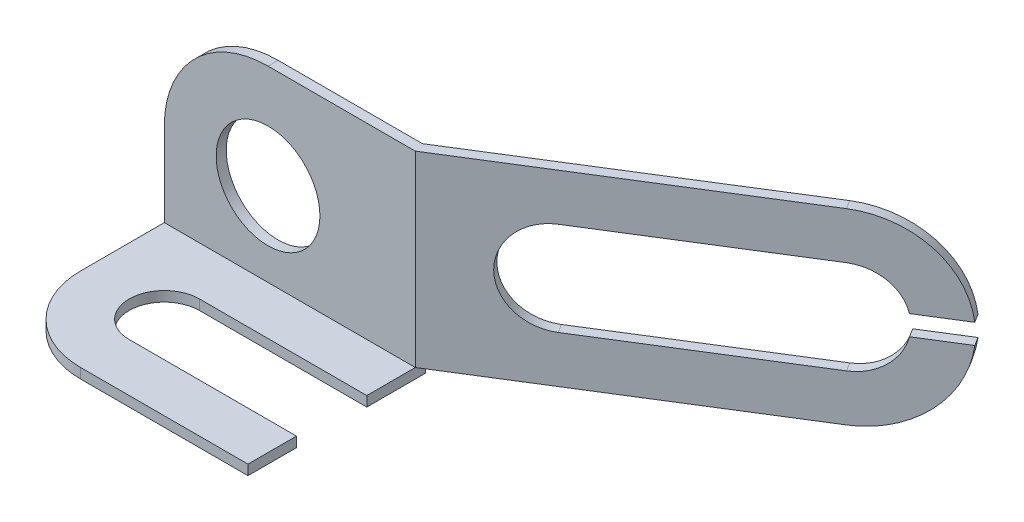
ISO-10303-21;
HEADER;
FILE_DESCRIPTION(('STEP AP214'),'2;1');
FILE_NAME('part.step','',(''),(''),'','','');
FILE_SCHEMA(('AUTOMOTIVE_DESIGN { 1 0 10303 214 1 1 1 1 }'));
ENDSEC;
DATA;
#1=APPLICATION_CONTEXT('core data for automotive mechanical design processes');
#2=APPLICATION_PROTOCOL_DEFINITION('international standard','automotive_design',2000,#1);
#3=PRODUCT_CONTEXT('',#1,'mechanical');
#4=PRODUCT('Part','Part','',(#3));
#5=PRODUCT_RELATED_PRODUCT_CATEGORY('part','',(#4));
#6=PRODUCT_DEFINITION_FORMATION('','',#4);
#7=PRODUCT_DEFINITION_CONTEXT('part definition',#1,'design');
#8=PRODUCT_DEFINITION('design','',#6,#7);
#9=PRODUCT_DEFINITION_SHAPE('','',#8);
#10=(LENGTH_UNIT() NAMED_UNIT(*) SI_UNIT(.MILLI.,.METRE.));
#11=(NAMED_UNIT(*) PLANE_ANGLE_UNIT() SI_UNIT($,.RADIAN.));
#12=(NAMED_UNIT(*) SI_UNIT($,.STERADIAN.) SOLID_ANGLE_UNIT());
#13=UNCERTAINTY_MEASURE_WITH_UNIT(LENGTH_MEASURE(1.E-05),#10,'distance_accuracy_value','');
#14=(GEOMETRIC_REPRESENTATION_CONTEXT(3) GLOBAL_UNCERTAINTY_ASSIGNED_CONTEXT((#13)) GLOBAL_UNIT_ASSIGNED_CONTEXT((#10,
#11,#12)) REPRESENTATION_CONTEXT('',''));
#15=CARTESIAN_POINT('',(0.,0.,0.));
#16=DIRECTION('',(0.,0.,1.));
#17=DIRECTION('',(1.,0.,0.));
#18=AXIS2_PLACEMENT_3D('',#15,#16,#17);
#19=CARTESIAN_POINT('',(1.55405478395852,0.56,-1.04183190988548));
#20=DIRECTION('',(0.529919264233206,0.,0.848048096156425));
#21=DIRECTION('',(0.848048096156426,0.,-0.529919264233206));
#22=AXIS2_PLACEMENT_3D('',#19,#20,#21);
#23=CYLINDRICAL_SURFACE('',#22,0.56);
#24=CARTESIAN_POINT('',(1.55405478395852,0.56,-1.04183190988548));
#25=DIRECTION('',(0.529919264233206,0.,0.848048096156425));
#26=DIRECTION('',(0.848048096156426,0.,-0.529919264233206));
#27=AXIS2_PLACEMENT_3D('',#24,#25,#26);
#28=CIRCLE('',#27,0.56);
#29=CARTESIAN_POINT('',(2.02622798073308,0.5,-1.33687846934296));
#30=VERTEX_POINT('',#29);
#31=CARTESIAN_POINT('',(1.55405478395852,0.,-1.04183190988548));
#32=VERTEX_POINT('',#31);
#33=EDGE_CURVE('E48',#30,#32,#28,.F.);
#34=ORIENTED_EDGE('',*,*,#33,.F.);
#35=DIRECTION('',(0.529919264233206,0.,0.848048096156425));
#36=VECTOR('',#35,1.);
#37=CARTESIAN_POINT('',(2.02622798073308,0.5,-1.33687846934295));
#38=LINE('',#37,#36);
#39=CARTESIAN_POINT('',(2.05802313658707,0.5,-1.28599558357357));
#40=VERTEX_POINT('',#39);
#41=EDGE_CURVE('E93',#30,#40,#38,.T.);
#42=ORIENTED_EDGE('',*,*,#41,.T.);
#43=CARTESIAN_POINT('',(1.58584993981252,0.56,-0.990949024116095));
#44=DIRECTION('',(0.529919264233206,0.,0.848048096156425));
#45=DIRECTION('',(0.848048096156426,0.,-0.529919264233206));
#46=AXIS2_PLACEMENT_3D('',#43,#44,#45);
#47=CIRCLE('',#46,0.56);
#48=CARTESIAN_POINT('',(1.58584993981251,0.,-0.990949024116095));
#49=VERTEX_POINT('',#48);
#50=EDGE_CURVE('E12',#49,#40,#47,.T.);
#51=ORIENTED_EDGE('',*,*,#50,.F.);
#52=DIRECTION('',(0.529919264233206,0.,0.848048096156425));
#53=VECTOR('',#52,1.);
#54=CARTESIAN_POINT('',(1.55405478395852,0.,-1.04183190988548));
#55=LINE('',#54,#53);
#56=EDGE_CURVE('E226',#32,#49,#55,.T.);
#57=ORIENTED_EDGE('',*,*,#56,.F.);
#58=EDGE_LOOP('',(#34,#42,#51,#57));
#59=FACE_BOUND('',#58,.T.);
#60=ADVANCED_FACE('F43',(#59),#23,.T.);
#61=CARTESIAN_POINT('',(-0.0317951558539923,0.,-0.0508828857693855));
#62=DIRECTION('',(-0.529919264233206,0.,-0.848048096156426));
#63=DIRECTION('',(-0.848048096156425,0.,0.529919264233206));
#64=AXIS2_PLACEMENT_3D('',#61,#62,#63);
#65=PLANE('',#64);
#66=CARTESIAN_POINT('',(1.55405478395852,0.56,-1.04183190988548));
#67=DIRECTION('',(0.529919264233206,0.,0.848048096156425));
#68=DIRECTION('',(0.848048096156426,0.,-0.529919264233206));
#69=AXIS2_PLACEMENT_3D('',#66,#67,#68);
#70=CIRCLE('',#69,0.56);
#71=CARTESIAN_POINT('',(1.55405478395852,1.12,-1.04183190988548));
#72=VERTEX_POINT('',#71);
#73=CARTESIAN_POINT('',(2.02622798073308,0.62,-1.33687846934296));
#74=VERTEX_POINT('',#73);
#75=EDGE_CURVE('E224',#72,#74,#70,.F.);
#76=ORIENTED_EDGE('',*,*,#75,.T.);
#77=DIRECTION('',(-0.848048096156425,0.,0.529919264233206));
#78=VECTOR('',#77,1.);
#79=CARTESIAN_POINT('',(1.78599244991624,0.62,-1.18676264889584));
#80=LINE('',#79,#78);
#81=CARTESIAN_POINT('',(1.78599244991624,0.62,-1.18676264889584));
#82=VERTEX_POINT('',#81);
#83=EDGE_CURVE('E247',#74,#82,#80,.T.);
#84=ORIENTED_EDGE('',*,*,#83,.T.);
#85=CARTESIAN_POINT('',(1.55405478395852,0.56,-1.04183190988548));
#86=DIRECTION('',(0.529919264233206,0.,0.848048096156425));
#87=DIRECTION('',(0.848048096156426,0.,-0.529919264233206));
#88=AXIS2_PLACEMENT_3D('',#85,#86,#87);
#89=CIRCLE('',#88,0.28);
#90=CARTESIAN_POINT('',(1.55405478395852,0.84,-1.04183190988548));
#91=VERTEX_POINT('',#90);
#92=EDGE_CURVE('E580',#82,#91,#89,.T.);
#93=ORIENTED_EDGE('',*,*,#92,.T.);
#94=DIRECTION('',(-0.848048096156425,0.,0.529919264233206));
#95=VECTOR('',#94,1.);
#96=CARTESIAN_POINT('',(1.55405478395852,0.84,-1.04183190988548));
#97=LINE('',#96,#95);
#98=CARTESIAN_POINT('',(0.493994663762991,0.84,-0.379432829593973));
#99=VERTEX_POINT('',#98);
#100=EDGE_CURVE('E579',#91,#99,#97,.T.);
#101=ORIENTED_EDGE('',*,*,#100,.T.);
#102=CARTESIAN_POINT('',(0.493994663762991,0.56,-0.379432829593973));
#103=DIRECTION('',(0.529919264233206,0.,0.848048096156425));
#104=DIRECTION('',(0.848048096156426,0.,-0.529919264233206));
#105=AXIS2_PLACEMENT_3D('',#102,#103,#104);
#106=CIRCLE('',#105,0.28);
#107=CARTESIAN_POINT('',(0.493994663762991,0.28,-0.379432829593973));
#108=VERTEX_POINT('',#107);
#109=EDGE_CURVE('E585',#99,#108,#106,.T.);
#110=ORIENTED_EDGE('',*,*,#109,.T.);
#111=DIRECTION('',(0.848048096156425,0.,-0.529919264233206));
#112=VECTOR('',#111,1.);
#113=CARTESIAN_POINT('',(1.55405478395852,0.28,-1.04183190988548));
#114=LINE('',#113,#112);
#115=CARTESIAN_POINT('',(1.55405478395852,0.28,-1.04183190988548));
#116=VERTEX_POINT('',#115);
#117=EDGE_CURVE('E587',#108,#116,#114,.T.);
#118=ORIENTED_EDGE('',*,*,#117,.T.);
#119=CARTESIAN_POINT('',(1.55405478395852,0.56,-1.04183190988548));
#120=DIRECTION('',(0.529919264233206,0.,0.848048096156425));
#121=DIRECTION('',(0.848048096156426,0.,-0.529919264233206));
#122=AXIS2_PLACEMENT_3D('',#119,#120,#121);
#123=CIRCLE('',#122,0.28);
#124=CARTESIAN_POINT('',(1.78599244991624,0.5,-1.18676264889584));
#125=VERTEX_POINT('',#124);
#126=EDGE_CURVE('E577',#116,#125,#123,.T.);
#127=ORIENTED_EDGE('',*,*,#126,.T.);
#128=DIRECTION('',(0.848048096156425,0.,-0.529919264233206));
#129=VECTOR('',#128,1.);
#130=CARTESIAN_POINT('',(1.78599244991624,0.5,-1.18676264889584));
#131=LINE('',#130,#129);
#132=EDGE_CURVE('E223',#125,#30,#131,.T.);
#133=ORIENTED_EDGE('',*,*,#132,.T.);
#134=ORIENTED_EDGE('',*,*,#33,.T.);
#135=DIRECTION('',(-0.848048096156425,0.,0.529919264233206));
#136=VECTOR('',#135,1.);
#137=CARTESIAN_POINT('',(-0.0317951558539923,0.,-0.0508828857693855));
#138=LINE('',#137,#136);
#139=CARTESIAN_POINT('',(-0.0172047231455286,0.,-0.06));
#140=VERTEX_POINT('',#139);
#141=EDGE_CURVE('E216',#32,#140,#138,.T.);
#142=ORIENTED_EDGE('',*,*,#141,.T.);
#143=DIRECTION('',(0.,-1.,0.));
#144=VECTOR('',#143,1.);
#145=CARTESIAN_POINT('',(-0.0172047231455285,0.,-0.06));
#146=LINE('',#145,#144);
#147=CARTESIAN_POINT('',(-0.0172047231455286,1.12,-0.06));
#148=VERTEX_POINT('',#147);
#149=EDGE_CURVE('E320',#148,#140,#146,.T.);
#150=ORIENTED_EDGE('',*,*,#149,.F.);
#151=DIRECTION('',(0.848048096156425,0.,-0.529919264233206));
#152=VECTOR('',#151,1.);
#153=CARTESIAN_POINT('',(-0.0317951558539923,1.12,-0.0508828857693857));
#154=LINE('',#153,#152);
#155=EDGE_CURVE('E240',#148,#72,#154,.T.);
#156=ORIENTED_EDGE('',*,*,#155,.T.);
#157=EDGE_LOOP('',(#76,#84,#93,#101,#110,#118,#127,#133,#134,#142,#150,#156));
#158=FACE_BOUND('',#157,.T.);
#159=ADVANCED_FACE('F217',(#158),#65,.T.);
#160=CARTESIAN_POINT('',(0.,0.,0.));
#161=DIRECTION('',(-0.529919264233206,0.,-0.848048096156426));
#162=DIRECTION('',(-0.848048096156425,0.,0.529919264233206));
#163=AXIS2_PLACEMENT_3D('',#160,#161,#162);
#164=PLANE('',#163);
#165=DIRECTION('',(-0.848048096156425,0.,0.529919264233206));
#166=VECTOR('',#165,1.);
#167=CARTESIAN_POINT('',(1.81778760577023,0.62,-1.13587976312645));
#168=LINE('',#167,#166);
#169=CARTESIAN_POINT('',(2.05802313658707,0.62,-1.28599558357357));
#170=VERTEX_POINT('',#169);
#171=CARTESIAN_POINT('',(1.81778760577023,0.62,-1.13587976312645));
#172=VERTEX_POINT('',#171);
#173=EDGE_CURVE('E64',#170,#172,#168,.T.);
#174=ORIENTED_EDGE('',*,*,#173,.F.);
#175=CARTESIAN_POINT('',(1.58584993981252,0.56,-0.990949024116095));
#176=DIRECTION('',(0.529919264233206,0.,0.848048096156425));
#177=DIRECTION('',(0.848048096156426,0.,-0.529919264233206));
#178=AXIS2_PLACEMENT_3D('',#175,#176,#177);
#179=CIRCLE('',#178,0.56);
#180=CARTESIAN_POINT('',(1.58584993981252,1.12,-0.990949024116095));
#181=VERTEX_POINT('',#180);
#182=EDGE_CURVE('E53',#170,#181,#179,.T.);
#183=ORIENTED_EDGE('',*,*,#182,.T.);
#184=DIRECTION('',(0.848048096156425,0.,-0.529919264233206));
#185=VECTOR('',#184,1.);
#186=CARTESIAN_POINT('',(0.,1.12,0.));
#187=LINE('',#186,#185);
#188=CARTESIAN_POINT('',(0.,1.12,0.));
#189=VERTEX_POINT('',#188);
#190=EDGE_CURVE('E258',#189,#181,#187,.T.);
#191=ORIENTED_EDGE('',*,*,#190,.F.);
#192=DIRECTION('',(0.,1.,0.));
#193=VECTOR('',#192,1.);
#194=CARTESIAN_POINT('',(0.,-0.06,0.));
#195=LINE('',#194,#193);
#196=CARTESIAN_POINT('',(0.,0.,0.));
#197=VERTEX_POINT('',#196);
#198=EDGE_CURVE('E294',#197,#189,#195,.T.);
#199=ORIENTED_EDGE('',*,*,#198,.F.);
#200=DIRECTION('',(-0.848048096156425,0.,0.529919264233206));
#201=VECTOR('',#200,1.);
#202=CARTESIAN_POINT('',(0.,0.,0.));
#203=LINE('',#202,#201);
#204=EDGE_CURVE('E245',#49,#197,#203,.T.);
#205=ORIENTED_EDGE('',*,*,#204,.F.);
#206=ORIENTED_EDGE('',*,*,#50,.T.);
#207=DIRECTION('',(0.848048096156425,0.,-0.529919264233206));
#208=VECTOR('',#207,1.);
#209=CARTESIAN_POINT('',(1.81778760577023,0.5,-1.13587976312645));
#210=LINE('',#209,#208);
#211=CARTESIAN_POINT('',(1.81778760577023,0.5,-1.13587976312645));
#212=VERTEX_POINT('',#211);
#213=EDGE_CURVE('E565',#212,#40,#210,.T.);
#214=ORIENTED_EDGE('',*,*,#213,.F.);
#215=CARTESIAN_POINT('',(1.58584993981252,0.56,-0.990949024116095));
#216=DIRECTION('',(0.529919264233206,0.,0.848048096156425));
#217=DIRECTION('',(0.848048096156426,0.,-0.529919264233206));
#218=AXIS2_PLACEMENT_3D('',#215,#216,#217);
#219=CIRCLE('',#218,0.28);
#220=CARTESIAN_POINT('',(1.58584993981251,0.28,-0.990949024116095));
#221=VERTEX_POINT('',#220);
#222=EDGE_CURVE('E562',#221,#212,#219,.T.);
#223=ORIENTED_EDGE('',*,*,#222,.F.);
#224=DIRECTION('',(0.848048096156425,0.,-0.529919264233206));
#225=VECTOR('',#224,1.);
#226=CARTESIAN_POINT('',(1.58584993981251,0.28,-0.990949024116095));
#227=LINE('',#226,#225);
#228=CARTESIAN_POINT('',(0.525789819616983,0.28,-0.328549943824587));
#229=VERTEX_POINT('',#228);
#230=EDGE_CURVE('E600',#229,#221,#227,.T.);
#231=ORIENTED_EDGE('',*,*,#230,.F.);
#232=CARTESIAN_POINT('',(0.525789819616983,0.56,-0.328549943824587));
#233=DIRECTION('',(0.529919264233206,0.,0.848048096156425));
#234=DIRECTION('',(0.848048096156426,0.,-0.529919264233206));
#235=AXIS2_PLACEMENT_3D('',#232,#233,#234);
#236=CIRCLE('',#235,0.28);
#237=CARTESIAN_POINT('',(0.525789819616983,0.84,-0.328549943824587));
#238=VERTEX_POINT('',#237);
#239=EDGE_CURVE('E592',#238,#229,#236,.T.);
#240=ORIENTED_EDGE('',*,*,#239,.F.);
#241=DIRECTION('',(-0.848048096156425,0.,0.529919264233206));
#242=VECTOR('',#241,1.);
#243=CARTESIAN_POINT('',(1.58584993981251,0.84,-0.990949024116095));
#244=LINE('',#243,#242);
#245=CARTESIAN_POINT('',(1.58584993981251,0.84,-0.990949024116095));
#246=VERTEX_POINT('',#245);
#247=EDGE_CURVE('E575',#246,#238,#244,.T.);
#248=ORIENTED_EDGE('',*,*,#247,.F.);
#249=CARTESIAN_POINT('',(1.58584993981252,0.56,-0.990949024116095));
#250=DIRECTION('',(0.529919264233206,0.,0.848048096156425));
#251=DIRECTION('',(0.848048096156426,0.,-0.529919264233206));
#252=AXIS2_PLACEMENT_3D('',#249,#250,#251);
#253=CIRCLE('',#252,0.28);
#254=EDGE_CURVE('E569',#172,#246,#253,.T.);
#255=ORIENTED_EDGE('',*,*,#254,.F.);
#256=EDGE_LOOP('',(#174,#183,#191,#199,#205,#206,#214,#223,#231,#240,#248,#255));
#257=FACE_BOUND('',#256,.T.);
#258=ADVANCED_FACE('F423',(#257),#164,.F.);
#259=DIRECTION('',(0.529919264233206,0.,0.848048096156425));
#260=VECTOR('',#259,1.);
#261=CARTESIAN_POINT('',(2.02622798073308,0.62,-1.33687846934295));
#262=LINE('',#261,#260);
#263=EDGE_CURVE('E257',#74,#170,#262,.T.);
#264=ORIENTED_EDGE('',*,*,#263,.F.);
#265=ORIENTED_EDGE('',*,*,#75,.F.);
#266=DIRECTION('',(-0.529919264233206,0.,-0.848048096156425));
#267=VECTOR('',#266,1.);
#268=CARTESIAN_POINT('',(1.55405478395852,1.12,-1.04183190988548));
#269=LINE('',#268,#267);
#270=EDGE_CURVE('E228',#181,#72,#269,.T.);
#271=ORIENTED_EDGE('',*,*,#270,.F.);
#272=ORIENTED_EDGE('',*,*,#182,.F.);
#273=EDGE_LOOP('',(#264,#265,#271,#272));
#274=FACE_BOUND('',#273,.T.);
#275=ADVANCED_FACE('F46',(#274),#23,.T.);
#276=CARTESIAN_POINT('',(0.,-0.06,-0.06));
#277=DIRECTION('',(1.,0.,0.));
#278=DIRECTION('',(0.,0.,-1.));
#279=AXIS2_PLACEMENT_3D('',#276,#277,#278);
#280=PLANE('',#279);
#281=DIRECTION('',(0.,1.,0.));
#282=VECTOR('',#281,1.);
#283=CARTESIAN_POINT('',(0.,-0.06,0.29));
#284=LINE('',#283,#282);
#285=CARTESIAN_POINT('',(0.,-0.06,0.29));
#286=VERTEX_POINT('',#285);
#287=CARTESIAN_POINT('',(0.,0.,0.29));
#288=VERTEX_POINT('',#287);
#289=EDGE_CURVE('E233',#286,#288,#284,.T.);
#290=ORIENTED_EDGE('',*,*,#289,.F.);
#291=DIRECTION('',(0.,0.,1.));
#292=VECTOR('',#291,1.);
#293=CARTESIAN_POINT('',(0.,-0.06,-0.06));
#294=LINE('',#293,#292);
#295=CARTESIAN_POINT('',(0.,-0.06,-0.06));
#296=VERTEX_POINT('',#295);
#297=EDGE_CURVE('E313',#296,#286,#294,.T.);
#298=ORIENTED_EDGE('',*,*,#297,.F.);
#299=DIRECTION('',(0.,1.,0.));
#300=VECTOR('',#299,1.);
#301=CARTESIAN_POINT('',(0.,-0.06,-0.06));
#302=LINE('',#301,#300);
#303=CARTESIAN_POINT('',(0.,0.,-0.06));
#304=VERTEX_POINT('',#303);
#305=EDGE_CURVE('E298',#296,#304,#302,.T.);
#306=ORIENTED_EDGE('',*,*,#305,.T.);
#307=DIRECTION('',(0.,0.,1.));
#308=VECTOR('',#307,1.);
#309=CARTESIAN_POINT('',(0.,0.,-0.06));
#310=LINE('',#309,#308);
#311=EDGE_CURVE('E237',#304,#197,#310,.T.);
#312=ORIENTED_EDGE('',*,*,#311,.T.);
#313=DIRECTION('',(0.,0.,-1.));
#314=VECTOR('',#313,1.);
#315=CARTESIAN_POINT('',(0.,0.,0.));
#316=LINE('',#315,#314);
#317=EDGE_CURVE('E280',#288,#197,#316,.T.);
#318=ORIENTED_EDGE('',*,*,#317,.F.);
#319=EDGE_LOOP('',(#290,#298,#306,#312,#318));
#320=FACE_BOUND('',#319,.T.);
#321=ADVANCED_FACE('F356',(#320),#280,.T.);
#322=CARTESIAN_POINT('',(0.,-0.06,-0.06));
#323=DIRECTION('',(0.,-1.,0.));
#324=DIRECTION('',(1.,0.,0.));
#325=AXIS2_PLACEMENT_3D('',#322,#323,#324);
#326=PLANE('',#325);
#327=ORIENTED_EDGE('',*,*,#297,.T.);
#328=DIRECTION('',(-1.,0.,0.));
#329=VECTOR('',#328,1.);
#330=CARTESIAN_POINT('',(-1.,-0.06,0.29));
#331=LINE('',#330,#329);
#332=CARTESIAN_POINT('',(-1.,-0.06,0.29));
#333=VERTEX_POINT('',#332);
#334=EDGE_CURVE('E345',#286,#333,#331,.T.);
#335=ORIENTED_EDGE('',*,*,#334,.T.);
#336=CARTESIAN_POINT('',(-1.,-0.06,0.5));
#337=DIRECTION('',(0.,1.,0.));
#338=DIRECTION('',(0.,0.,1.));
#339=AXIS2_PLACEMENT_3D('',#336,#337,#338);
#340=CIRCLE('',#339,0.21);
#341=CARTESIAN_POINT('',(-1.,-0.06,0.71));
#342=VERTEX_POINT('',#341);
#343=EDGE_CURVE('E394',#333,#342,#340,.T.);
#344=ORIENTED_EDGE('',*,*,#343,.T.);
#345=DIRECTION('',(1.,0.,0.));
#346=VECTOR('',#345,1.);
#347=CARTESIAN_POINT('',(-1.,-0.06,0.71));
#348=LINE('',#347,#346);
#349=CARTESIAN_POINT('',(0.,-0.06,0.71));
#350=VERTEX_POINT('',#349);
#351=EDGE_CURVE('E383',#342,#350,#348,.T.);
#352=ORIENTED_EDGE('',*,*,#351,.T.);
#353=CARTESIAN_POINT('',(0.,-0.06,1.));
#354=VERTEX_POINT('',#353);
#355=EDGE_CURVE('E319',#350,#354,#294,.T.);
#356=ORIENTED_EDGE('',*,*,#355,.T.);
#357=DIRECTION('',(1.,0.,0.));
#358=VECTOR('',#357,1.);
#359=CARTESIAN_POINT('',(0.,-0.06,1.));
#360=LINE('',#359,#358);
#361=CARTESIAN_POINT('',(-1.,-0.06,1.));
#362=VERTEX_POINT('',#361);
#363=EDGE_CURVE('E279',#362,#354,#360,.T.);
#364=ORIENTED_EDGE('',*,*,#363,.F.);
#365=CARTESIAN_POINT('',(-1.,-0.0600000000000001,0.5));
#366=DIRECTION('',(0.,-1.,0.));
#367=DIRECTION('',(1.,0.,0.));
#368=AXIS2_PLACEMENT_3D('',#365,#366,#367);
#369=CIRCLE('',#368,0.5);
#370=CARTESIAN_POINT('',(-1.5,-0.0600000000000002,0.5));
#371=VERTEX_POINT('',#370);
#372=EDGE_CURVE('E331',#362,#371,#369,.T.);
#373=ORIENTED_EDGE('',*,*,#372,.T.);
#374=DIRECTION('',(0.,0.,1.));
#375=VECTOR('',#374,1.);
#376=CARTESIAN_POINT('',(-1.5,-0.0600000000000002,-0.06));
#377=LINE('',#376,#375);
#378=CARTESIAN_POINT('',(-1.5,-0.0600000000000002,-0.06));
#379=VERTEX_POINT('',#378);
#380=EDGE_CURVE('E310',#379,#371,#377,.T.);
#381=ORIENTED_EDGE('',*,*,#380,.F.);
#382=DIRECTION('',(1.,0.,0.));
#383=VECTOR('',#382,1.);
#384=CARTESIAN_POINT('',(0.,-0.06,-0.06));
#385=LINE('',#384,#383);
#386=EDGE_CURVE('E302',#379,#296,#385,.T.);
#387=ORIENTED_EDGE('',*,*,#386,.T.);
#388=EDGE_LOOP('',(#327,#335,#344,#352,#356,#364,#373,#381,#387));
#389=FACE_BOUND('',#388,.T.);
#390=ADVANCED_FACE('F379',(#389),#326,.T.);
#391=CARTESIAN_POINT('',(0.,0.,0.));
#392=DIRECTION('',(0.,-1.,0.));
#393=DIRECTION('',(0.,0.,-1.));
#394=AXIS2_PLACEMENT_3D('',#391,#392,#393);
#395=PLANE('',#394);
#396=DIRECTION('',(1.,0.,0.));
#397=VECTOR('',#396,1.);
#398=CARTESIAN_POINT('',(-1.,0.,0.71));
#399=LINE('',#398,#397);
#400=CARTESIAN_POINT('',(-1.,0.,0.71));
#401=VERTEX_POINT('',#400);
#402=CARTESIAN_POINT('',(0.,0.,0.71));
#403=VERTEX_POINT('',#402);
#404=EDGE_CURVE('E388',#401,#403,#399,.T.);
#405=ORIENTED_EDGE('',*,*,#404,.F.);
#406=CARTESIAN_POINT('',(-1.,0.,0.5));
#407=DIRECTION('',(0.,1.,0.));
#408=DIRECTION('',(0.,0.,1.));
#409=AXIS2_PLACEMENT_3D('',#406,#407,#408);
#410=CIRCLE('',#409,0.21);
#411=CARTESIAN_POINT('',(-1.,0.,0.29));
#412=VERTEX_POINT('',#411);
#413=EDGE_CURVE('E358',#412,#401,#410,.T.);
#414=ORIENTED_EDGE('',*,*,#413,.F.);
#415=DIRECTION('',(-1.,0.,0.));
#416=VECTOR('',#415,1.);
#417=CARTESIAN_POINT('',(-1.,0.,0.29));
#418=LINE('',#417,#416);
#419=EDGE_CURVE('E339',#288,#412,#418,.T.);
#420=ORIENTED_EDGE('',*,*,#419,.F.);
#421=ORIENTED_EDGE('',*,*,#317,.T.);
#422=DIRECTION('',(-1.,0.,0.));
#423=VECTOR('',#422,1.);
#424=CARTESIAN_POINT('',(0.,0.,0.));
#425=LINE('',#424,#423);
#426=CARTESIAN_POINT('',(-1.5,0.,0.));
#427=VERTEX_POINT('',#426);
#428=EDGE_CURVE('E286',#197,#427,#425,.T.);
#429=ORIENTED_EDGE('',*,*,#428,.T.);
#430=DIRECTION('',(0.,0.,1.));
#431=VECTOR('',#430,1.);
#432=CARTESIAN_POINT('',(-1.5,0.,0.));
#433=LINE('',#432,#431);
#434=CARTESIAN_POINT('',(-1.5,0.,0.5));
#435=VERTEX_POINT('',#434);
#436=EDGE_CURVE('E287',#427,#435,#433,.T.);
#437=ORIENTED_EDGE('',*,*,#436,.T.);
#438=CARTESIAN_POINT('',(-1.,0.,0.5));
#439=DIRECTION('',(0.,-1.,0.));
#440=DIRECTION('',(0.,0.,-1.));
#441=AXIS2_PLACEMENT_3D('',#438,#439,#440);
#442=CIRCLE('',#441,0.5);
#443=CARTESIAN_POINT('',(-1.,0.,1.));
#444=VERTEX_POINT('',#443);
#445=EDGE_CURVE('E329',#435,#444,#442,.F.);
#446=ORIENTED_EDGE('',*,*,#445,.T.);
#447=DIRECTION('',(1.,0.,0.));
#448=VECTOR('',#447,1.);
#449=CARTESIAN_POINT('',(0.,0.,1.));
#450=LINE('',#449,#448);
#451=CARTESIAN_POINT('',(0.,0.,1.));
#452=VERTEX_POINT('',#451);
#453=EDGE_CURVE('E284',#444,#452,#450,.T.);
#454=ORIENTED_EDGE('',*,*,#453,.T.);
#455=EDGE_CURVE('E282',#452,#403,#316,.T.);
#456=ORIENTED_EDGE('',*,*,#455,.T.);
#457=EDGE_LOOP('',(#405,#414,#420,#421,#429,#437,#446,#454,#456));
#458=FACE_BOUND('',#457,.T.);
#459=ADVANCED_FACE('F352',(#458),#395,.F.);
#460=DIRECTION('',(0.,-1.,0.));
#461=VECTOR('',#460,1.);
#462=CARTESIAN_POINT('',(0.,-0.06,0.71));
#463=LINE('',#462,#461);
#464=EDGE_CURVE('E338',#403,#350,#463,.T.);
#465=ORIENTED_EDGE('',*,*,#464,.F.);
#466=ORIENTED_EDGE('',*,*,#455,.F.);
#467=DIRECTION('',(0.,1.,0.));
#468=VECTOR('',#467,1.);
#469=CARTESIAN_POINT('',(0.,-0.06,1.));
#470=LINE('',#469,#468);
#471=EDGE_CURVE('E283',#354,#452,#470,.T.);
#472=ORIENTED_EDGE('',*,*,#471,.F.);
#473=ORIENTED_EDGE('',*,*,#355,.F.);
#474=EDGE_LOOP('',(#465,#466,#472,#473));
#475=FACE_BOUND('',#474,.T.);
#476=ADVANCED_FACE('F389',(#475),#280,.T.);
#477=CARTESIAN_POINT('',(0.,0.,-0.06));
#478=DIRECTION('',(0.,0.,1.));
#479=DIRECTION('',(1.,0.,0.));
#480=AXIS2_PLACEMENT_3D('',#477,#478,#479);
#481=PLANE('',#480);
#482=CARTESIAN_POINT('',(-0.88,0.5,-0.06));
#483=DIRECTION('',(0.,0.,1.));
#484=DIRECTION('',(1.,0.,0.));
#485=AXIS2_PLACEMENT_3D('',#482,#483,#484);
#486=CIRCLE('',#485,0.31);
#487=CARTESIAN_POINT('',(-0.57,0.5,-0.06));
#488=VERTEX_POINT('',#487);
#489=EDGE_CURVE('E262',#488,#488,#486,.T.);
#490=ORIENTED_EDGE('',*,*,#489,.T.);
#491=EDGE_LOOP('',(#490));
#492=FACE_BOUND('',#491,.T.);
#493=DIRECTION('',(0.,-1.,0.));
#494=VECTOR('',#493,1.);
#495=CARTESIAN_POINT('',(-1.5,-0.0600000000000002,-0.06));
#496=LINE('',#495,#494);
#497=CARTESIAN_POINT('',(-1.5,0.5,-0.06));
#498=VERTEX_POINT('',#497);
#499=EDGE_CURVE('E305',#498,#379,#496,.T.);
#500=ORIENTED_EDGE('',*,*,#499,.F.);
#501=CARTESIAN_POINT('',(-0.88,0.5,-0.06));
#502=DIRECTION('',(0.,0.,1.));
#503=DIRECTION('',(1.,0.,0.));
#504=AXIS2_PLACEMENT_3D('',#501,#502,#503);
#505=CIRCLE('',#504,0.62);
#506=CARTESIAN_POINT('',(-0.88,1.12,-0.06));
#507=VERTEX_POINT('',#506);
#508=EDGE_CURVE('E204',#498,#507,#505,.F.);
#509=ORIENTED_EDGE('',*,*,#508,.T.);
#510=DIRECTION('',(-1.,0.,0.));
#511=VECTOR('',#510,1.);
#512=CARTESIAN_POINT('',(0.,1.12,-0.06));
#513=LINE('',#512,#511);
#514=EDGE_CURVE('E299',#148,#507,#513,.T.);
#515=ORIENTED_EDGE('',*,*,#514,.F.);
#516=ORIENTED_EDGE('',*,*,#149,.T.);
#517=DIRECTION('',(-1.,0.,0.));
#518=VECTOR('',#517,1.);
#519=CARTESIAN_POINT('',(0.,0.,-0.06));
#520=LINE('',#519,#518);
#521=EDGE_CURVE('E232',#304,#140,#520,.T.);
#522=ORIENTED_EDGE('',*,*,#521,.F.);
#523=ORIENTED_EDGE('',*,*,#305,.F.);
#524=ORIENTED_EDGE('',*,*,#386,.F.);
#525=EDGE_LOOP('',(#500,#509,#515,#516,#522,#523,#524));
#526=FACE_BOUND('',#525,.T.);
#527=ADVANCED_FACE('F402',(#492,#526),#481,.F.);
#528=CARTESIAN_POINT('',(-1.5,-0.0600000000000002,-0.06));
#529=DIRECTION('',(-1.,0.,0.));
#530=DIRECTION('',(0.,0.,1.));
#531=AXIS2_PLACEMENT_3D('',#528,#529,#530);
#532=PLANE('',#531);
#533=ORIENTED_EDGE('',*,*,#380,.T.);
#534=DIRECTION('',(0.,1.,0.));
#535=VECTOR('',#534,1.);
#536=CARTESIAN_POINT('',(-1.5,-0.0600000000000002,0.5));
#537=LINE('',#536,#535);
#538=EDGE_CURVE('E321',#371,#435,#537,.T.);
#539=ORIENTED_EDGE('',*,*,#538,.T.);
#540=ORIENTED_EDGE('',*,*,#436,.F.);
#541=DIRECTION('',(0.,-1.,0.));
#542=VECTOR('',#541,1.);
#543=CARTESIAN_POINT('',(-1.5,-0.0600000000000002,0.));
#544=LINE('',#543,#542);
#545=CARTESIAN_POINT('',(-1.5,0.5,0.));
#546=VERTEX_POINT('',#545);
#547=EDGE_CURVE('E297',#546,#427,#544,.T.);
#548=ORIENTED_EDGE('',*,*,#547,.F.);
#549=DIRECTION('',(0.,0.,1.));
#550=VECTOR('',#549,1.);
#551=CARTESIAN_POINT('',(-1.5,0.5,-0.06));
#552=LINE('',#551,#550);
#553=EDGE_CURVE('E325',#546,#498,#552,.F.);
#554=ORIENTED_EDGE('',*,*,#553,.T.);
#555=ORIENTED_EDGE('',*,*,#499,.T.);
#556=EDGE_LOOP('',(#533,#539,#540,#548,#554,#555));
#557=FACE_BOUND('',#556,.T.);
#558=ADVANCED_FACE('F370',(#557),#532,.T.);
#559=CARTESIAN_POINT('',(0.,1.12,-0.06));
#560=DIRECTION('',(0.,1.,0.));
#561=DIRECTION('',(-1.,0.,0.));
#562=AXIS2_PLACEMENT_3D('',#559,#560,#561);
#563=PLANE('',#562);
#564=ORIENTED_EDGE('',*,*,#190,.T.);
#565=ORIENTED_EDGE('',*,*,#270,.T.);
#566=ORIENTED_EDGE('',*,*,#155,.F.);
#567=ORIENTED_EDGE('',*,*,#514,.T.);
#568=DIRECTION('',(0.,0.,1.));
#569=VECTOR('',#568,1.);
#570=CARTESIAN_POINT('',(-0.88,1.12,-0.06));
#571=LINE('',#570,#569);
#572=CARTESIAN_POINT('',(-0.88,1.12,0.));
#573=VERTEX_POINT('',#572);
#574=EDGE_CURVE('E333',#507,#573,#571,.T.);
#575=ORIENTED_EDGE('',*,*,#574,.T.);
#576=DIRECTION('',(-1.,0.,0.));
#577=VECTOR('',#576,1.);
#578=CARTESIAN_POINT('',(0.,1.12,0.));
#579=LINE('',#578,#577);
#580=EDGE_CURVE('E309',#189,#573,#579,.T.);
#581=ORIENTED_EDGE('',*,*,#580,.F.);
#582=EDGE_LOOP('',(#564,#565,#566,#567,#575,#581));
#583=FACE_BOUND('',#582,.T.);
#584=ADVANCED_FACE('F259',(#583),#563,.T.);
#585=CARTESIAN_POINT('',(0.,0.,0.));
#586=DIRECTION('',(0.,0.,1.));
#587=DIRECTION('',(1.,0.,0.));
#588=AXIS2_PLACEMENT_3D('',#585,#586,#587);
#589=PLANE('',#588);
#590=CARTESIAN_POINT('',(-0.88,0.5,0.));
#591=DIRECTION('',(0.,0.,1.));
#592=DIRECTION('',(1.,0.,0.));
#593=AXIS2_PLACEMENT_3D('',#590,#591,#592);
#594=CIRCLE('',#593,0.31);
#595=CARTESIAN_POINT('',(-0.57,0.5,0.));
#596=VERTEX_POINT('',#595);
#597=EDGE_CURVE('E261',#596,#596,#594,.T.);
#598=ORIENTED_EDGE('',*,*,#597,.F.);
#599=EDGE_LOOP('',(#598));
#600=FACE_BOUND('',#599,.T.);
#601=ORIENTED_EDGE('',*,*,#580,.T.);
#602=CARTESIAN_POINT('',(-0.88,0.5,0.));
#603=DIRECTION('',(0.,0.,1.));
#604=DIRECTION('',(1.,0.,0.));
#605=AXIS2_PLACEMENT_3D('',#602,#603,#604);
#606=CIRCLE('',#605,0.62);
#607=EDGE_CURVE('E337',#573,#546,#606,.T.);
#608=ORIENTED_EDGE('',*,*,#607,.T.);
#609=ORIENTED_EDGE('',*,*,#547,.T.);
#610=ORIENTED_EDGE('',*,*,#428,.F.);
#611=ORIENTED_EDGE('',*,*,#198,.T.);
#612=EDGE_LOOP('',(#601,#608,#609,#610,#611));
#613=FACE_BOUND('',#612,.T.);
#614=ADVANCED_FACE('F365',(#600,#613),#589,.T.);
#615=CARTESIAN_POINT('',(0.,-0.06,1.));
#616=DIRECTION('',(0.,0.,1.));
#617=DIRECTION('',(1.,0.,0.));
#618=AXIS2_PLACEMENT_3D('',#615,#616,#617);
#619=PLANE('',#618);
#620=ORIENTED_EDGE('',*,*,#453,.F.);
#621=DIRECTION('',(0.,1.,0.));
#622=VECTOR('',#621,1.);
#623=CARTESIAN_POINT('',(-1.,-0.06,1.));
#624=LINE('',#623,#622);
#625=EDGE_CURVE('E330',#444,#362,#624,.F.);
#626=ORIENTED_EDGE('',*,*,#625,.T.);
#627=ORIENTED_EDGE('',*,*,#363,.T.);
#628=ORIENTED_EDGE('',*,*,#471,.T.);
#629=EDGE_LOOP('',(#620,#626,#627,#628));
#630=FACE_BOUND('',#629,.T.);
#631=ADVANCED_FACE('F380',(#630),#619,.T.);
#632=CARTESIAN_POINT('',(-0.0317951558539923,0.,-0.0508828857693855));
#633=DIRECTION('',(0.,1.,0.));
#634=DIRECTION('',(0.,0.,1.));
#635=AXIS2_PLACEMENT_3D('',#632,#633,#634);
#636=PLANE('',#635);
#637=ORIENTED_EDGE('',*,*,#141,.F.);
#638=ORIENTED_EDGE('',*,*,#56,.T.);
#639=ORIENTED_EDGE('',*,*,#204,.T.);
#640=ORIENTED_EDGE('',*,*,#311,.F.);
#641=ORIENTED_EDGE('',*,*,#521,.T.);
#642=EDGE_LOOP('',(#637,#638,#639,#640,#641));
#643=FACE_BOUND('',#642,.T.);
#644=ADVANCED_FACE('F231',(#643),#636,.F.);
#645=CARTESIAN_POINT('',(-1.,-0.0600000000000002,0.5));
#646=DIRECTION('',(0.,1.,0.));
#647=DIRECTION('',(0.,0.,1.));
#648=AXIS2_PLACEMENT_3D('',#645,#646,#647);
#649=CYLINDRICAL_SURFACE('',#648,0.5);
#650=ORIENTED_EDGE('',*,*,#372,.F.);
#651=ORIENTED_EDGE('',*,*,#625,.F.);
#652=ORIENTED_EDGE('',*,*,#445,.F.);
#653=ORIENTED_EDGE('',*,*,#538,.F.);
#654=EDGE_LOOP('',(#650,#651,#652,#653));
#655=FACE_BOUND('',#654,.T.);
#656=ADVANCED_FACE('F373',(#655),#649,.T.);
#657=CARTESIAN_POINT('',(-0.88,0.5,-0.06));
#658=DIRECTION('',(0.,0.,1.));
#659=DIRECTION('',(1.,0.,0.));
#660=AXIS2_PLACEMENT_3D('',#657,#658,#659);
#661=CYLINDRICAL_SURFACE('',#660,0.62);
#662=ORIENTED_EDGE('',*,*,#508,.F.);
#663=ORIENTED_EDGE('',*,*,#553,.F.);
#664=ORIENTED_EDGE('',*,*,#607,.F.);
#665=ORIENTED_EDGE('',*,*,#574,.F.);
#666=EDGE_LOOP('',(#662,#663,#664,#665));
#667=FACE_BOUND('',#666,.T.);
#668=ADVANCED_FACE('F404',(#667),#661,.T.);
#669=CARTESIAN_POINT('',(-0.88,0.5,-0.06));
#670=DIRECTION('',(0.,0.,1.));
#671=DIRECTION('',(1.,0.,0.));
#672=AXIS2_PLACEMENT_3D('',#669,#670,#671);
#673=CYLINDRICAL_SURFACE('',#672,0.31);
#674=ORIENTED_EDGE('',*,*,#489,.F.);
#675=EDGE_LOOP('',(#674));
#676=FACE_BOUND('',#675,.T.);
#677=ORIENTED_EDGE('',*,*,#597,.T.);
#678=EDGE_LOOP('',(#677));
#679=FACE_BOUND('',#678,.T.);
#680=ADVANCED_FACE('F407',(#676,#679),#673,.F.);
#681=CARTESIAN_POINT('',(-1.,-0.06,0.5));
#682=DIRECTION('',(0.,1.,0.));
#683=DIRECTION('',(0.,0.,1.));
#684=AXIS2_PLACEMENT_3D('',#681,#682,#683);
#685=CYLINDRICAL_SURFACE('',#684,0.21);
#686=ORIENTED_EDGE('',*,*,#413,.T.);
#687=DIRECTION('',(0.,1.,0.));
#688=VECTOR('',#687,1.);
#689=CARTESIAN_POINT('',(-1.,-0.06,0.71));
#690=LINE('',#689,#688);
#691=EDGE_CURVE('E275',#342,#401,#690,.T.);
#692=ORIENTED_EDGE('',*,*,#691,.F.);
#693=ORIENTED_EDGE('',*,*,#343,.F.);
#694=DIRECTION('',(0.,1.,0.));
#695=VECTOR('',#694,1.);
#696=CARTESIAN_POINT('',(-1.,-0.06,0.29));
#697=LINE('',#696,#695);
#698=EDGE_CURVE('E212',#333,#412,#697,.T.);
#699=ORIENTED_EDGE('',*,*,#698,.T.);
#700=EDGE_LOOP('',(#686,#692,#693,#699));
#701=FACE_BOUND('',#700,.T.);
#702=ADVANCED_FACE('F414',(#701),#685,.F.);
#703=CARTESIAN_POINT('',(-1.,-0.06,0.29));
#704=DIRECTION('',(0.,0.,-1.));
#705=DIRECTION('',(-1.,0.,0.));
#706=AXIS2_PLACEMENT_3D('',#703,#704,#705);
#707=PLANE('',#706);
#708=ORIENTED_EDGE('',*,*,#289,.T.);
#709=ORIENTED_EDGE('',*,*,#419,.T.);
#710=ORIENTED_EDGE('',*,*,#698,.F.);
#711=ORIENTED_EDGE('',*,*,#334,.F.);
#712=EDGE_LOOP('',(#708,#709,#710,#711));
#713=FACE_BOUND('',#712,.T.);
#714=ADVANCED_FACE('F348',(#713),#707,.F.);
#715=CARTESIAN_POINT('',(-1.,-0.06,0.71));
#716=DIRECTION('',(0.,0.,1.));
#717=DIRECTION('',(1.,0.,0.));
#718=AXIS2_PLACEMENT_3D('',#715,#716,#717);
#719=PLANE('',#718);
#720=ORIENTED_EDGE('',*,*,#464,.T.);
#721=ORIENTED_EDGE('',*,*,#351,.F.);
#722=ORIENTED_EDGE('',*,*,#691,.T.);
#723=ORIENTED_EDGE('',*,*,#404,.T.);
#724=EDGE_LOOP('',(#720,#721,#722,#723));
#725=FACE_BOUND('',#724,.T.);
#726=ADVANCED_FACE('F469',(#725),#719,.F.);
#727=CARTESIAN_POINT('',(1.55405478395852,0.56,-1.04183190988548));
#728=DIRECTION('',(0.529919264233206,0.,0.848048096156425));
#729=DIRECTION('',(0.848048096156426,0.,-0.529919264233206));
#730=AXIS2_PLACEMENT_3D('',#727,#728,#729);
#731=CYLINDRICAL_SURFACE('',#730,0.28);
#732=ORIENTED_EDGE('',*,*,#222,.T.);
#733=DIRECTION('',(0.529919264233206,0.,0.848048096156425));
#734=VECTOR('',#733,1.);
#735=CARTESIAN_POINT('',(1.78599244991624,0.5,-1.18676264889584));
#736=LINE('',#735,#734);
#737=EDGE_CURVE('E105',#125,#212,#736,.T.);
#738=ORIENTED_EDGE('',*,*,#737,.F.);
#739=ORIENTED_EDGE('',*,*,#126,.F.);
#740=DIRECTION('',(0.529919264233206,0.,0.848048096156425));
#741=VECTOR('',#740,1.);
#742=CARTESIAN_POINT('',(1.55405478395852,0.28,-1.04183190988548));
#743=LINE('',#742,#741);
#744=EDGE_CURVE('E391',#116,#221,#743,.T.);
#745=ORIENTED_EDGE('',*,*,#744,.T.);
#746=EDGE_LOOP('',(#732,#738,#739,#745));
#747=FACE_BOUND('',#746,.T.);
#748=ADVANCED_FACE('F478',(#747),#731,.F.);
#749=CARTESIAN_POINT('',(1.55405478395852,0.28,-1.04183190988548));
#750=DIRECTION('',(0.,-1.,0.));
#751=DIRECTION('',(1.,0.,0.));
#752=AXIS2_PLACEMENT_3D('',#749,#750,#751);
#753=PLANE('',#752);
#754=ORIENTED_EDGE('',*,*,#230,.T.);
#755=ORIENTED_EDGE('',*,*,#744,.F.);
#756=ORIENTED_EDGE('',*,*,#117,.F.);
#757=DIRECTION('',(0.529919264233206,0.,0.848048096156425));
#758=VECTOR('',#757,1.);
#759=CARTESIAN_POINT('',(0.493994663762991,0.28,-0.379432829593973));
#760=LINE('',#759,#758);
#761=EDGE_CURVE('E602',#108,#229,#760,.T.);
#762=ORIENTED_EDGE('',*,*,#761,.T.);
#763=EDGE_LOOP('',(#754,#755,#756,#762));
#764=FACE_BOUND('',#763,.T.);
#765=ADVANCED_FACE('F501',(#764),#753,.F.);
#766=CARTESIAN_POINT('',(0.493994663762991,0.56,-0.379432829593973));
#767=DIRECTION('',(0.529919264233206,0.,0.848048096156425));
#768=DIRECTION('',(0.848048096156426,0.,-0.529919264233206));
#769=AXIS2_PLACEMENT_3D('',#766,#767,#768);
#770=CYLINDRICAL_SURFACE('',#769,0.28);
#771=ORIENTED_EDGE('',*,*,#239,.T.);
#772=ORIENTED_EDGE('',*,*,#761,.F.);
#773=ORIENTED_EDGE('',*,*,#109,.F.);
#774=DIRECTION('',(0.529919264233206,0.,0.848048096156425));
#775=VECTOR('',#774,1.);
#776=CARTESIAN_POINT('',(0.493994663762991,0.84,-0.379432829593973));
#777=LINE('',#776,#775);
#778=EDGE_CURVE('E604',#99,#238,#777,.T.);
#779=ORIENTED_EDGE('',*,*,#778,.T.);
#780=EDGE_LOOP('',(#771,#772,#773,#779));
#781=FACE_BOUND('',#780,.T.);
#782=ADVANCED_FACE('F509',(#781),#770,.F.);
#783=CARTESIAN_POINT('',(1.55405478395852,0.84,-1.04183190988548));
#784=DIRECTION('',(0.,1.,0.));
#785=DIRECTION('',(-1.,0.,0.));
#786=AXIS2_PLACEMENT_3D('',#783,#784,#785);
#787=PLANE('',#786);
#788=ORIENTED_EDGE('',*,*,#247,.T.);
#789=ORIENTED_EDGE('',*,*,#778,.F.);
#790=ORIENTED_EDGE('',*,*,#100,.F.);
#791=DIRECTION('',(0.529919264233206,0.,0.848048096156425));
#792=VECTOR('',#791,1.);
#793=CARTESIAN_POINT('',(1.55405478395852,0.84,-1.04183190988548));
#794=LINE('',#793,#792);
#795=EDGE_CURVE('E603',#91,#246,#794,.T.);
#796=ORIENTED_EDGE('',*,*,#795,.T.);
#797=EDGE_LOOP('',(#788,#789,#790,#796));
#798=FACE_BOUND('',#797,.T.);
#799=ADVANCED_FACE('F518',(#798),#787,.F.);
#800=CARTESIAN_POINT('',(1.55405478395852,0.56,-1.04183190988548));
#801=DIRECTION('',(0.529919264233206,0.,0.848048096156425));
#802=DIRECTION('',(0.848048096156426,0.,-0.529919264233206));
#803=AXIS2_PLACEMENT_3D('',#800,#801,#802);
#804=CYLINDRICAL_SURFACE('',#803,0.28);
#805=ORIENTED_EDGE('',*,*,#254,.T.);
#806=ORIENTED_EDGE('',*,*,#795,.F.);
#807=ORIENTED_EDGE('',*,*,#92,.F.);
#808=DIRECTION('',(0.529919264233206,0.,0.848048096156425));
#809=VECTOR('',#808,1.);
#810=CARTESIAN_POINT('',(1.78599244991624,0.62,-1.18676264889584));
#811=LINE('',#810,#809);
#812=EDGE_CURVE('E609',#82,#172,#811,.T.);
#813=ORIENTED_EDGE('',*,*,#812,.T.);
#814=EDGE_LOOP('',(#805,#806,#807,#813));
#815=FACE_BOUND('',#814,.T.);
#816=ADVANCED_FACE('F529',(#815),#804,.F.);
#817=CARTESIAN_POINT('',(1.78599244991624,0.62,-1.18676264889584));
#818=DIRECTION('',(0.,1.,0.));
#819=DIRECTION('',(0.,0.,1.));
#820=AXIS2_PLACEMENT_3D('',#817,#818,#819);
#821=PLANE('',#820);
#822=ORIENTED_EDGE('',*,*,#173,.T.);
#823=ORIENTED_EDGE('',*,*,#812,.F.);
#824=ORIENTED_EDGE('',*,*,#83,.F.);
#825=ORIENTED_EDGE('',*,*,#263,.T.);
#826=EDGE_LOOP('',(#822,#823,#824,#825));
#827=FACE_BOUND('',#826,.T.);
#828=ADVANCED_FACE('F538',(#827),#821,.F.);
#829=CARTESIAN_POINT('',(1.78599244991624,0.5,-1.18676264889584));
#830=DIRECTION('',(0.,-1.,0.));
#831=DIRECTION('',(0.,0.,-1.));
#832=AXIS2_PLACEMENT_3D('',#829,#830,#831);
#833=PLANE('',#832);
#834=ORIENTED_EDGE('',*,*,#213,.T.);
#835=ORIENTED_EDGE('',*,*,#41,.F.);
#836=ORIENTED_EDGE('',*,*,#132,.F.);
#837=ORIENTED_EDGE('',*,*,#737,.T.);
#838=EDGE_LOOP('',(#834,#835,#836,#837));
#839=FACE_BOUND('',#838,.T.);
#840=ADVANCED_FACE('F549',(#839),#833,.F.);
#841=CLOSED_SHELL('',(#60,#159,#258,#275,#321,#390,#459,#476,#527,#558,#584,#614,#631,#644,#656,
#668,#680,#702,#714,#726,#748,#765,#782,#799,#816,#828,#840));
#842=MANIFOLD_SOLID_BREP('B2',#841);
#843=ADVANCED_BREP_SHAPE_REPRESENTATION('',(#18,#842),#14);
#844=SHAPE_DEFINITION_REPRESENTATION(#9,#843);
ENDSEC;
END-ISO-10303-21;
